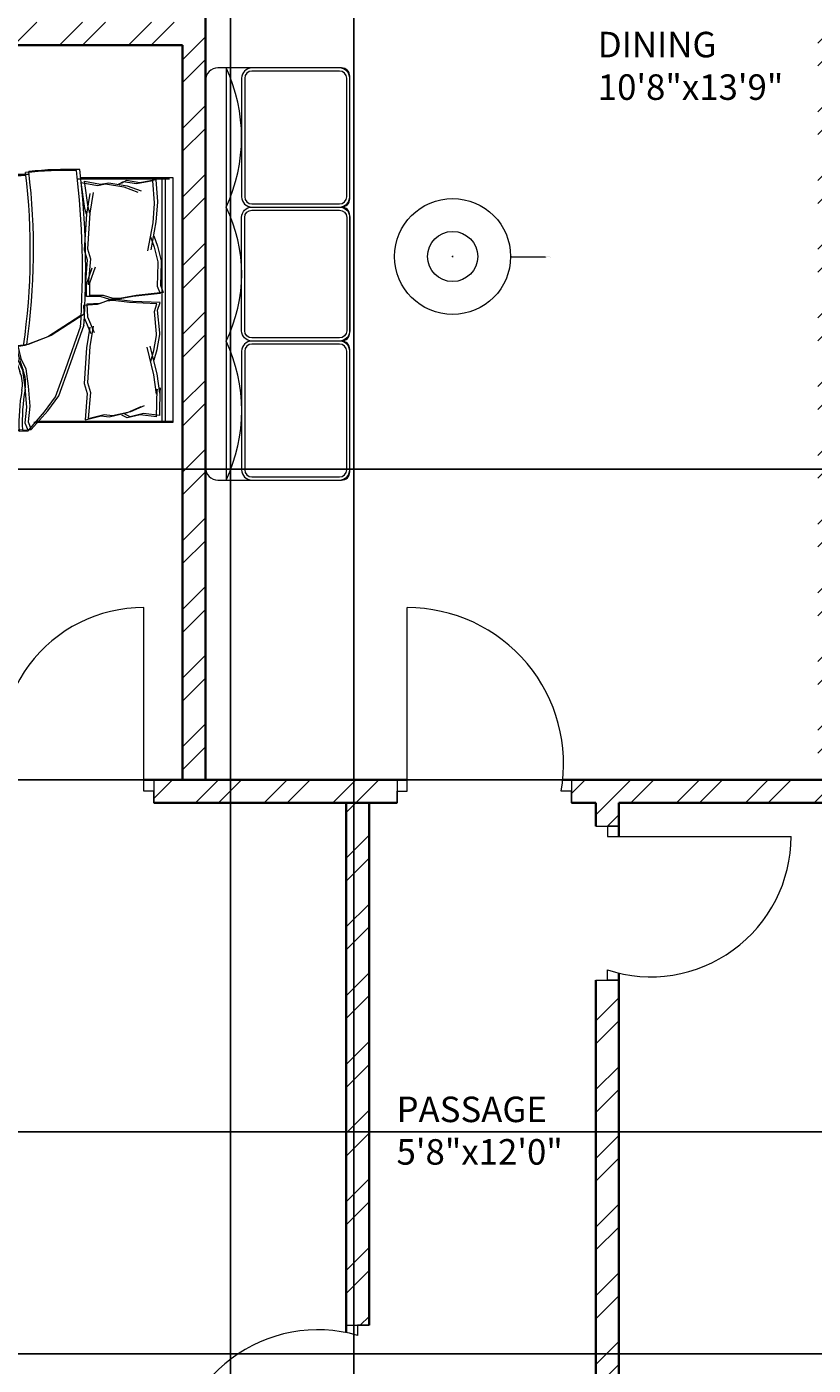
# Model space of a CAD drawing. Units: inches. Extents: x 1965 to 2673, y 1802 to 2669.
# Tile 8 of 16: x 2218 to 2372, y 2154 to 2416. Entities that reach past the tile are written whole.
import ezdxf

# ---------------------------------------------------------------- set-up
doc = ezdxf.new("R2010")
doc.units = ezdxf.units.IN
for name, color, linetype, lineweight in [('A-ANNO-DIMS', 2, 'Continuous', 18), ('A-AREA-IDEN', 7, 'Continuous', 18), ('A-DOOR', 11, 'Continuous', 18), ('A-FURN', 8, 'Continuous', 13), ('A-WALL', 7, 'Continuous', 35), ('A-WALL-PATT', 252, 'Continuous', 13)]:
    doc.layers.add(name, color=color, linetype=linetype, lineweight=lineweight)
doc.styles.get("Standard").update_dxf_attribs({"font": 'arial.ttf'})
doc.dimstyles.get("Standard").update_dxf_attribs({"dimtxt": 0.18, "dimasz": 0.18, "dimexe": 0.18, "dimexo": 0.0625, "dimgap": 0.09, "dimtad": 0, "dimtih": 1, "dimtoh": 1, "dimdec": 4, "dimzin": 0, "dimdsep": 46, "dimtxsty": 'Standard', "dimcen": 0.09, "dimadec": 0, "dimazin": 0, "dimtfac": 1, "dimtdec": 4, "dimtofl": 0, "dimtmove": 0, "dimatfit": 3, "dimfxl": 1, "dimtolj": 1, "dimtzin": 0, "dimarcsym": 0})

# ---------------------------------------------------------------- blocks, each defined once
blk = doc.blocks.new('BED-DOUBLE')
for p, q in [((3.47, 63.33), (3.47, 81.44)), ((3.47, 63.33), (3.47, 81.44)), ((3.47, 81.44), (51.49, 81.44)), ((51.26, 81.44), (51.26, 54.83)), ((51.26, 81.44), (51.26, 54.83)), ((51.49, 81.44), (51.49, 80.8)), ((3.47, 79.91), (51.26, 79.91)), ((3.47, 79.91), (51.26, 79.91)), ((3.7, 62.69), (3.7, 80.8)), ((3.7, 62.69), (3.7, 80.8)), ((3.7, 79.27), (51.49, 79.27)), ((3.7, 79.27), (51.49, 79.27)), ((16.87, 78.41), (19.76, 79.14)), ((16.87, 78.41), (19.76, 79.14)), ((19.76, 79.14), (20.09, 79.14)), ((19.76, 79.14), (20.09, 79.14)), ((20.09, 79.14), (24.53, 78.99)), ((20.09, 79.14), (24.53, 78.99)), ((24.53, 78.99), (25.98, 79.57)), ((24.53, 78.99), (25.98, 79.57)), ((24.76, 78.35), (26.21, 78.93)), ((24.76, 78.35), (26.21, 78.93)), ((25.98, 79.57), (26.56, 74.22)), ((25.98, 79.57), (26.56, 74.22)), ((26.21, 78.93), (26.78, 73.58)), ((26.21, 78.93), (26.78, 73.58)), ((27.97, 78.95), (27.73, 73.57)), ((27.97, 78.95), (27.73, 73.57)), ((29.45, 78.46), (27.97, 78.95)), ((29.45, 78.46), (27.97, 78.95)), ((33.88, 78.88), (29.45, 78.46)), ((33.88, 78.88), (29.45, 78.46)), ((34.2, 78.9), (33.88, 78.88)), ((34.2, 78.9), (33.88, 78.88)), ((37.13, 78.36), (34.2, 78.9)), ((37.13, 78.36), (34.2, 78.9)), ((45.71, 78.9), (41.91, 78.37)), ((45.71, 78.9), (41.91, 78.37)), ((50.11, 78.88), (44.7, 78.98)), ((44.7, 78.98), (45.71, 78.9)), ((50.11, 78.88), (44.7, 78.98)), ((44.7, 78.98), (45.71, 78.9)), ((50.11, 78.88), (49.73, 75.67)), ((50.11, 78.88), (49.73, 75.67)), ((51.49, 80.8), (51.49, 54.19)), ((51.49, 80.8), (51.49, 54.19)), ((3.89, 78.1), (8.17, 78.43)), ((3.89, 78.1), (8.17, 78.43)), ((3.89, 78.12), (4.47, 74.94)), ((3.89, 78.12), (4.47, 74.94)), ((4.12, 77.46), (8.4, 77.79)), ((4.12, 77.46), (8.4, 77.79)), ((4.12, 77.49), (4.7, 74.3)), ((4.12, 77.49), (4.7, 74.3)), ((8.17, 78.43), (8.28, 78.41)), ((8.17, 78.43), (8.28, 78.41)), ((8.28, 78.41), (12.1, 78.12)), ((8.28, 78.41), (12.1, 78.12)), ((8.4, 77.79), (8.51, 77.77)), ((8.4, 77.79), (8.51, 77.77)), ((8.51, 77.77), (12.33, 77.49)), ((8.51, 77.77), (12.33, 77.49)), ((12.1, 78.12), (17.6, 77.11)), ((12.1, 78.12), (17.6, 77.11)), ((12.33, 77.49), (17.82, 76.47)), ((12.33, 77.49), (17.82, 76.47)), ((14.85, 77.69), (16.87, 78.41)), ((14.85, 77.69), (16.87, 78.41)), ((15.08, 77.05), (17.1, 77.77)), ((15.08, 77.05), (17.1, 77.77)), ((17.1, 77.77), (19.99, 78.5)), ((17.1, 77.77), (19.99, 78.5)), ((19.99, 78.5), (20.31, 78.5)), ((19.99, 78.5), (20.31, 78.5)), ((20.31, 78.5), (24.76, 78.35)), ((20.31, 78.5), (24.76, 78.35)), ((28.2, 78.31), (27.96, 72.93)), ((28.2, 78.31), (27.96, 72.93)), ((29.68, 77.82), (28.2, 78.31)), ((29.68, 77.82), (28.2, 78.31)), ((34.11, 78.24), (29.68, 77.82)), ((34.11, 78.24), (29.68, 77.82)), ((34.43, 78.26), (34.11, 78.24)), ((34.43, 78.26), (34.11, 78.24)), ((37.36, 77.72), (34.43, 78.26)), ((37.36, 77.72), (34.43, 78.26)), ((41.91, 78.37), (36.49, 77.02)), ((41.91, 78.37), (36.49, 77.02)), ((42.14, 77.73), (36.72, 76.38)), ((42.14, 77.73), (36.72, 76.38)), ((39.2, 77.77), (37.13, 78.36)), ((39.19, 77.77), (37.13, 78.36)), ((39.42, 77.13), (37.36, 77.72)), ((39.42, 77.13), (37.36, 77.72)), ((45.94, 78.26), (42.14, 77.73)), ((45.94, 78.26), (42.14, 77.73)), ((50.34, 78.24), (44.93, 78.34)), ((44.93, 78.34), (45.94, 78.26)), ((50.34, 78.24), (44.93, 78.34)), ((44.93, 78.34), (45.94, 78.26)), ((50.34, 78.24), (49.96, 75.03)), ((50.34, 78.24), (49.96, 75.03)), ((4.47, 74.94), (4.03, 72.34)), ((4.47, 74.94), (4.03, 72.34)), ((4.7, 74.3), (4.26, 71.7)), ((4.7, 74.3), (4.26, 71.7)), ((5.05, 72.49), (6.06, 75.23)), ((5.05, 72.49), (6.06, 75.23)), ((5.27, 71.85), (6.29, 74.59)), ((5.27, 71.85), (6.29, 74.59)), ((26.56, 74.22), (27.13, 71.04)), ((26.56, 74.22), (27.13, 71.04)), ((26.78, 73.58), (27.36, 70.4)), ((26.78, 73.58), (27.36, 70.4)), ((27.73, 73.57), (27.35, 70.36)), ((27.73, 73.57), (27.35, 70.36)), ((49.3, 73.18), (48.12, 75.86)), ((49.3, 73.18), (48.12, 75.86)), ((49.53, 72.54), (48.35, 75.22)), ((49.53, 72.54), (48.35, 75.22)), ((49.73, 75.67), (50.32, 73.1)), ((49.73, 75.67), (50.32, 73.1)), ((49.96, 75.03), (50.55, 72.46)), ((49.96, 75.03), (50.55, 72.46)), ((4.03, 72.34), (4.61, 71.33)), ((4.03, 72.34), (4.61, 71.33)), ((4.26, 71.7), (4.84, 70.69)), ((4.26, 71.7), (4.84, 70.69)), ((4.47, 68.87), (5.05, 72.49)), ((4.47, 68.87), (5.05, 72.49)), ((4.7, 68.23), (5.27, 71.85)), ((4.7, 68.23), (5.27, 71.85)), ((27.13, 71.04), (27.13, 69.74)), ((27.13, 71.04), (27.13, 69.74)), ((27.96, 72.93), (27.58, 69.72)), ((27.96, 72.93), (27.58, 69.72)), ((50.11, 69.61), (49.3, 73.18)), ((50.11, 69.61), (49.3, 73.18)), ((50.34, 68.97), (49.53, 72.54)), ((50.34, 68.97), (49.53, 72.54)), ((50.32, 73.1), (49.81, 72.06)), ((50.32, 73.1), (49.81, 72.06)), ((50.55, 72.46), (50.04, 71.42)), ((50.55, 72.46), (50.04, 71.42)), ((4.76, 67.28), (4.47, 68.87)), ((4.76, 67.28), (4.47, 68.87)), ((4.99, 66.64), (4.7, 68.23)), ((4.99, 66.64), (4.7, 68.23)), ((27.13, 69.74), (26.56, 67.86)), ((27.13, 69.74), (26.56, 67.86)), ((27.36, 69.1), (26.78, 67.22)), ((27.36, 69.1), (26.78, 67.22)), ((27.35, 70.36), (27.43, 69.06)), ((27.35, 70.36), (27.43, 69.06)), ((27.36, 70.4), (27.36, 69.1)), ((27.36, 70.4), (27.36, 69.1)), ((27.43, 69.06), (28.13, 67.22)), ((27.43, 69.06), (28.13, 67.22)), ((27.58, 69.72), (27.66, 68.42)), ((27.58, 69.72), (27.66, 68.42)), ((27.66, 68.42), (28.35, 66.58)), ((27.66, 68.42), (28.35, 66.58)), ((49.92, 68.01), (50.11, 69.61)), ((49.92, 68.01), (50.11, 69.61)), ((50.15, 67.37), (50.34, 68.97)), ((50.15, 67.37), (50.34, 68.97)), ((4.18, 64.1), (4.76, 67.28)), ((4.18, 64.1), (4.76, 67.28)), ((4.41, 63.46), (4.99, 66.64)), ((4.41, 63.46), (4.99, 66.64)), ((6.38, 65.81), (10.41, 65.15)), ((6.38, 65.81), (10.41, 65.15)), ((24.1, 65.18), (20.95, 66.27)), ((24.1, 65.18), (20.95, 66.27)), ((24.33, 64.54), (21.18, 65.63)), ((24.33, 64.54), (21.18, 65.63)), ((26.56, 67.86), (26.56, 65.18)), ((26.56, 67.86), (26.56, 65.18)), ((26.78, 67.22), (26.78, 64.54)), ((26.78, 67.22), (26.78, 64.54)), ((28.13, 67.22), (28.29, 64.55)), ((28.13, 67.22), (28.29, 64.55)), ((28.35, 66.58), (28.52, 63.91)), ((28.35, 66.58), (28.52, 63.91)), ((30.75, 64.7), (33.82, 65.99)), ((30.75, 64.7), (33.82, 65.99)), ((32.56, 65.81), (36.59, 65.15)), ((32.56, 65.81), (36.59, 65.15)), ((50.69, 64.87), (49.92, 68.01)), ((50.69, 64.87), (49.92, 68.01)), ((50.92, 64.23), (50.15, 67.37)), ((50.92, 64.23), (50.15, 67.37)), ((9.28, 64.82), (4.18, 64.1)), ((9.28, 64.82), (4.18, 64.1)), ((9.5, 64.18), (4.41, 63.46)), ((9.5, 64.18), (4.41, 63.46)), ((6.6, 65.17), (10.64, 64.51)), ((6.61, 65.17), (10.64, 64.51)), ((10.41, 65.15), (9.28, 64.82)), ((10.41, 65.15), (9.28, 64.82)), ((10.64, 64.51), (9.5, 64.18)), ((10.64, 64.51), (9.5, 64.18)), ((10.41, 65.15), (17.42, 64.71)), ((10.41, 65.15), (17.42, 64.71)), ((10.64, 64.51), (17.65, 64.08)), ((10.64, 64.51), (17.65, 64.08)), ((17.42, 64.71), (19.38, 65.27)), ((17.42, 64.71), (19.38, 65.27)), ((17.65, 64.08), (19.61, 64.63)), ((17.65, 64.08), (19.61, 64.63)), ((19.38, 65.27), (24.51, 64.87)), ((19.38, 65.27), (24.51, 64.87)), ((19.61, 64.63), (24.74, 64.23)), ((19.61, 64.63), (24.74, 64.23)), ((26.56, 65.18), (24.1, 65.18)), ((26.56, 65.18), (24.1, 65.18)), ((26.78, 64.54), (24.33, 64.54)), ((26.78, 64.54), (24.33, 64.54)), ((28.29, 64.55), (30.75, 64.7)), ((28.29, 64.55), (30.75, 64.7)), ((28.52, 63.91), (30.97, 64.06)), ((28.52, 63.91), (30.97, 64.06)), ((30.25, 64.06), (34.44, 57.56)), ((30.25, 64.06), (34.44, 57.56)), ((30.48, 63.42), (34.67, 56.92)), ((30.48, 63.42), (34.67, 56.92)), ((30.97, 64.06), (34.04, 65.35)), ((30.97, 64.06), (34.04, 65.35)), ((40.64, 61.12), (32.3, 64.06)), ((40.64, 61.12), (32.3, 64.06)), ((40.87, 60.48), (32.53, 63.42)), ((40.87, 60.48), (32.53, 63.42)), ((32.79, 65.17), (36.82, 64.51)), ((32.79, 65.17), (36.82, 64.51)), ((36.59, 65.15), (43.6, 64.71)), ((36.59, 65.15), (43.6, 64.71)), ((36.82, 64.51), (43.83, 64.08)), ((36.82, 64.51), (43.83, 64.08)), ((43.6, 64.71), (45.56, 65.27)), ((43.6, 64.71), (45.56, 65.27)), ((43.83, 64.08), (45.79, 64.63)), ((43.83, 64.08), (45.79, 64.63)), ((45.56, 65.27), (50.69, 64.87)), ((45.56, 65.27), (50.69, 64.87)), ((45.79, 64.63), (50.92, 64.23)), ((45.79, 64.63), (50.92, 64.23)), ((46.21, 59.11), (40.64, 61.12)), ((46.21, 59.11), (40.64, 61.12)), ((46.44, 58.47), (40.87, 60.48)), ((46.44, 58.47), (40.87, 60.48)), ((49.16, 56.95), (46.21, 59.11)), ((49.16, 56.95), (46.21, 59.11)), ((49.39, 56.31), (46.44, 58.47)), ((49.39, 56.31), (46.44, 58.47)), ((34.44, 57.56), (36.15, 53.08)), ((34.44, 57.56), (36.15, 53.08)), ((34.67, 56.92), (36.38, 52.44)), ((34.67, 56.92), (36.38, 52.44)), ((52.86, 53.69), (49.16, 56.95)), ((52.86, 53.69), (49.16, 56.95)), ((53.09, 53.06), (49.39, 56.31)), ((53.09, 53.06), (49.39, 56.31)), ((36.15, 53.08), (36.46, 51.06)), ((36.15, 53.08), (36.46, 51.06)), ((38.94, 51.68), (40.95, 52.61)), ((38.94, 51.68), (40.95, 52.61)), ((40.95, 52.61), (44.36, 53.08)), ((40.95, 52.61), (44.36, 53.08)), ((44.36, 53.08), (48.23, 53.39)), ((44.36, 53.08), (48.23, 53.39)), ((44.58, 52.44), (48.46, 52.75)), ((44.58, 52.44), (48.46, 52.75)), ((48.23, 53.39), (51.33, 53.08)), ((48.23, 53.39), (51.33, 53.08)), ((48.46, 52.75), (51.55, 52.44)), ((48.46, 52.75), (51.55, 52.44)), ((51.33, 53.08), (52.86, 53.69)), ((51.33, 53.08), (52.86, 53.69)), ((51.55, 52.44), (53.09, 53.06)), ((51.55, 52.44), (53.09, 53.06)), ((52.94, 51.95), (52.86, 53.69, 3.87)), ((52.94, 51.95), (52.86, 53.69, 3.87)), ((53.17, 51.31), (53.09, 53.06, 3.87)), ((53.17, 51.31), (53.09, 53.06, 3.87)), ((36.38, 52.44), (36.69, 50.42)), ((36.38, 52.44), (36.69, 50.42)), ((36.46, 51.06), (38.94, 51.68)), ((36.46, 51.06), (38.94, 51.68)), ((36.69, 50.42), (39.16, 51.04)), ((36.69, 50.42), (39.16, 51.04)), ((39.16, 51.04), (41.18, 51.97)), ((39.16, 51.04), (41.18, 51.97)), ((41.18, 51.97), (44.58, 52.44)), ((41.18, 51.97), (44.58, 52.44)), ((15.06, 2.2), (39.67, 2.2)), ((15.06, 2.2), (39.67, 2.2)), ((15.29, 1.56), (39.9, 1.56)), ((15.29, 1.56), (39.9, 1.56))]:
    blk.add_line(p, q)
for centre, radius, start, end in [((85.16, 61.34), 83.31, 178.7218, 185.604), ((85.16, 61.34), 83.31, 178.7218, 185.604), ((21.35, -100.61), 164.97, 86.0865, 96.7821), ((21.35, -100.61), 164.97, 86.0865, 96.7821), ((21.58, -101.25), 164.97, 86.0865, 96.7821), ((21.58, -101.25), 164.97, 86.0865, 96.7821), ((85.39, 60.71), 83.31, 178.7218, 185.604), ((85.38, 60.71), 83.31, 178.7218, 185.604), ((17.75, -74.88), 129.02, 81.7845, 96.9006), ((17.75, -74.88), 129.02, 81.7845, 96.9006), ((17.98, -75.51), 129.02, 81.7845, 96.9006), ((17.98, -75.51), 129.02, 81.7845, 96.9006), ((-167.31, 50.27), 170.11, 358.4762, 1.0082), ((-167.31, 50.27), 170.11, 358.4762, 1.0082), ((-167.08, 49.63), 170.11, 358.4762, 1.0082), ((-167.08, 49.63), 170.11, 358.4762, 1.0082), ((43.74, 46.37), 6.22, 78.6608, 113.7384), ((43.74, 46.37), 6.22, 78.6608, 113.7384), ((51.32, 88.1), 36.18, 259.8763, 272.5657), ((51.32, 88.1), 36.18, 259.8763, 272.5657), ((36.63, 51), 0.185, 160.2464, 271.1377), ((36.63, 51), 0.185, 160.2464, 271.1377), ((31.15, 79.96), 29.65, 280.6617, 289.8806), ((31.15, 79.96), 29.65, 280.6617, 289.8806), ((36.86, 50.36), 0.185, 160.2464, 271.1377), ((36.86, 50.36), 0.185, 160.2464, 271.1377), ((31.38, 79.32), 29.65, 280.6617, 289.8806), ((31.38, 79.32), 29.65, 280.6617, 289.8806), ((43.97, 45.74), 6.22, 78.6608, 113.7384), ((43.97, 45.74), 6.22, 78.6608, 113.7384), ((51.55, 87.46), 36.18, 259.8763, 272.5657), ((51.55, 87.46), 36.18, 259.8763, 272.5657), ((182.26, 45.13), 129.5, 176.9791, 183.8365), ((182.26, 45.13), 129.5, 176.9791, 183.8365), ((182.49, 44.49), 129.5, 176.9791, 183.8365), ((182.49, 44.49), 129.5, 176.9791, 183.8365), ((484.82, 30.83), 482.31, 178.2277, 181.7185), ((484.82, 30.83), 482.31, 178.2277, 181.7185), ((485.05, 30.19), 482.31, 178.2277, 181.7185), ((485.05, 30.19), 482.31, 178.2277, 181.7185), ((-4508.75, 13.62), 4561.86, 0.00217, 0.28689), ((-4508.75, 13.62), 4561.86, 0.00217, 0.28689), ((-4508.52, 12.98), 4561.86, 0.00217, 0.28689), ((-4508.52, 12.98), 4561.86, 0.00217, 0.28689), ((-26.9, 16.93), 29.63, 346.0648, 358.9113), ((-26.9, 16.93), 29.63, 346.0648, 358.9113), ((-26.68, 16.29), 29.63, 346.0648, 358.9113), ((-26.68, 16.29), 29.63, 346.0648, 358.9113), ((76.15, 12.77), 23.07, 177.4714, 206.4681), ((76.15, 12.77), 23.07, 177.4714, 206.4681), ((76.38, 12.14), 23.07, 177.4714, 206.4681), ((76.38, 12.14), 23.07, 177.4714, 206.4681), ((-21.66, 11.17), 23.56, 337.9751, 356.652), ((-21.66, 11.17), 23.56, 337.9751, 356.652), ((-21.44, 10.53), 23.56, 337.9751, 356.652), ((-21.44, 10.53), 23.56, 337.9751, 356.652), ((-17.23, 105.15), 106.46, 283.3832, 287.7053), ((-17.23, 105.15), 106.46, 283.3832, 287.7053), ((-17, 104.51), 106.46, 283.3832, 287.7053), ((-17, 104.51), 106.46, 283.3832, 287.7053), ((1.08, 1.72), 1.09, 146.1736, 293.4781), ((1.08, 1.72), 1.09, 146.1736, 293.4781), ((1.31, 1.08), 1.09, 146.1736, 293.4781), ((1.31, 1.08), 1.09, 146.1736, 293.4781), ((21.42, -119.4), 121.76, 92.9958, 99.4091), ((21.42, -119.4), 121.76, 92.9958, 99.4091), ((21.65, -120.04), 121.76, 92.9958, 99.4091), ((21.65, -120.04), 121.76, 92.9958, 99.4091), ((41.15, -130.84), 133.04, 84.4998, 90.6351), ((41.15, -130.84), 133.04, 84.4998, 90.6351), ((41.38, -131.48), 133.04, 84.4998, 90.6351), ((41.37, -131.48), 133.04, 84.4998, 90.6351), ((54.4, 2.57), 1.1, 242.6588, 356.02), ((54.4, 2.57), 1.1, 242.6588, 356.02), ((54.63, 1.93), 1.1, 242.6588, 356.02), ((54.63, 1.93), 1.1, 242.6588, 356.02)]:
    blk.add_arc(centre, radius, start, end)
blk = doc.blocks.new('*D47')
at = {"layer": 'A-ANNO-DIMS', "color": 0, "lineweight": -2, "transparency": 16777216}
for p, q in [((2573.53, 2199.58), (2012.19, 2199.58)), ((2012.37, 2199.4), (2012.37, 2178.02)), ((2012.37, 2156.27), (2012.37, 2177.65)), ((2573.53, 2156.09), (2012.19, 2156.09))]:
    blk.add_line(p, q, dxfattribs=at)
at = {"layer": 'A-ANNO-DIMS', "color": 0, "transparency": 16777216}
for points in [[(2012.34, 2199.4), (2012.4, 2199.4), (2012.37, 2199.58)], [(2012.34, 2156.27), (2012.4, 2156.27), (2012.37, 2156.09)]]:
    blk.add_solid(points, dxfattribs=at)
at = {"layer": 'Defpoints', "color": 0, "transparency": 16777216}
for p in [(2012.37, 2199.58), (2573.59, 2199.58), (2573.59, 2156.09)]:
    blk.add_point(p, dxfattribs=at)
at = {"layer": 'A-ANNO-DIMS', "color": 0, "transparency": 16777216, "insert": (2012.37, 2177.83), "char_height": 0.18, "attachment_point": 5}
blk.add_mtext('\\A1;43.48', dxfattribs=at)
blk = doc.blocks.new('*D48')
at = {"layer": 'A-ANNO-DIMS', "color": 0, "lineweight": -2, "transparency": 16777216}
for p, q in [((2573.53, 2329.47), (2012.19, 2329.47)), ((2012.37, 2329.29), (2012.37, 2299.21)), ((2012.37, 2268.77), (2012.37, 2298.85)), ((2573.53, 2268.59), (2012.19, 2268.59))]:
    blk.add_line(p, q, dxfattribs=at)
at = {"layer": 'A-ANNO-DIMS', "color": 0, "transparency": 16777216}
for points in [[(2012.34, 2329.29), (2012.4, 2329.29), (2012.37, 2329.47)], [(2012.34, 2268.77), (2012.4, 2268.77), (2012.37, 2268.59)]]:
    blk.add_solid(points, dxfattribs=at)
at = {"layer": 'Defpoints', "color": 0, "transparency": 16777216}
for p in [(2012.37, 2329.47), (2573.59, 2329.47), (2573.59, 2268.59)]:
    blk.add_point(p, dxfattribs=at)
at = {"layer": 'A-ANNO-DIMS', "color": 0, "transparency": 16777216, "insert": (2012.37, 2299.03), "char_height": 0.18, "attachment_point": 5}
blk.add_mtext('\\A1;60.87', dxfattribs=at)
blk = doc.blocks.new('*D53')
at = {"layer": 'A-ANNO-DIMS', "color": 0, "lineweight": -2, "transparency": 16777216}
for p, q in [((2257.52, 2457.53), (2257.52, 1838.49)), ((2281.66, 2457.53), (2281.66, 1838.49)), ((2257.7, 1838.67), (2269.12, 1838.67)), ((2281.48, 1838.67), (2270.05, 1838.67))]:
    blk.add_line(p, q, dxfattribs=at)
at = {"layer": 'A-ANNO-DIMS', "color": 0, "transparency": 16777216}
for points in [[(2257.7, 1838.7), (2257.7, 1838.64), (2257.52, 1838.67)], [(2281.48, 1838.7), (2281.48, 1838.64), (2281.66, 1838.67)]]:
    blk.add_solid(points, dxfattribs=at)
at = {"layer": 'Defpoints', "color": 0, "transparency": 16777216}
for p in [(2257.52, 2457.59), (2281.66, 2457.59), (2281.66, 1838.67)]:
    blk.add_point(p, dxfattribs=at)
at = {"layer": 'A-ANNO-DIMS', "color": 0, "transparency": 16777216, "insert": (2269.59, 1838.67), "char_height": 0.18, "attachment_point": 5}
blk.add_mtext('\\A1;24.145', dxfattribs=at)
blk = doc.blocks.new('*D55')
at = {"layer": 'A-ANNO-DIMS', "color": 0, "lineweight": -2, "transparency": 16777216}
for p, q in [((2300.93, 2371.16), (2301.11, 2371.16)), ((2301.02, 2371.07), (2301.02, 2371.25)), ((2319.19, 2371.06), (2312.55, 2371.1))]:
    blk.add_line(p, q, dxfattribs=at)
at = {"layer": 'A-ANNO-DIMS', "color": 0, "transparency": 16777216}
blk.add_solid([(2312.56, 2371.13), (2312.55, 2371.07), (2312.37, 2371.1)], dxfattribs=at)
at = {"layer": 'Defpoints', "color": 0, "transparency": 16777216}
for p in [(2289.66, 2371.22), (2312.37, 2371.1)]:
    blk.add_point(p, dxfattribs=at)
at = {"layer": 'A-ANNO-DIMS', "color": 0, "transparency": 16777216, "insert": (2319.75, 2371.06), "char_height": 0.18, "attachment_point": 5}
blk.add_mtext('\\A1;∅22.716', dxfattribs=at)

msp = doc.modelspace()

# ---------------------------------------------------------------- hatches: boundary and pattern name
at = {"layer": 'A-WALL-PATT'}
h = msp.add_hatch(dxfattribs=at)
h.set_pattern_fill('ANSI32', color=256)
h.paths.add_polyline_path([(2051.5927, 2561.0914), (2076.7559, 2561.0914), (2076.7559, 2563.3414), (2076.7559, 2565.5914), (2047.0927, 2565.5914), (2047.0927, 2518.3824), (2051.5927, 2518.3824)])
h.paths.add_polyline_path([(2051.5927, 2458.3824), (2049.3427, 2458.3824), (2047.0927, 2458.3824), (2047.0927, 2412.5914), (2248.0927, 2412.5914), (2248.0927, 2268.5914), (2252.5927, 2268.5914), (2252.5927, 2412.5914), (2252.5927, 2421.0404), (2250.3427, 2421.0404), (2248.0927, 2421.0404), (2248.0927, 2417.0914), (2051.5927, 2417.0914)])
h.paths.add_polyline_path([(2211.4933, 2268.5914), (2104.0927, 2268.5914), (2104.0927, 2272.4654), (2101.8427, 2272.4654), (2099.5927, 2272.4654), (2099.5927, 2268.5914), (2051.5927, 2268.5914), (2051.5927, 2264.0914), (2147.5927, 2264.0914), (2147.5927, 2259.8893), (2152.0927, 2259.8893), (2152.0927, 2264.0914), (2211.4933, 2264.0914), (2211.4933, 2266.3414)])
h.paths.add_polyline_path([(2104.0927, 2376.0914), (2099.5927, 2376.0914), (2047.0927, 2376.0914), (2047.0927, 2333.0682), (2051.5927, 2333.0682), (2051.5927, 2371.5914), (2099.5927, 2371.5914), (2099.5927, 2293.6123), (2104.0927, 2293.6123)], flags=17)
h.paths.add_polyline_path([(2051.5927, 2309.0682), (2047.0927, 2309.0682), (2047.0927, 2233.5821), (2051.5927, 2233.5821)])
h.paths.add_polyline_path([(2104.0927, 2412.5914), (2099.5927, 2412.5914), (2099.5927, 2376.0914), (2104.0927, 2376.0914)], flags=17)
h.paths.add_polyline_path([(2290.1254, 2268.5914), (2242.4924, 2268.5914), (2242.4924, 2264.0914), (2290.1254, 2264.0914), (2290.1254, 2266.3414)])
h.paths.add_polyline_path([(2284.653, 2264.0914), (2280.153, 2264.0914), (2280.153, 2161.6826), (2284.653, 2161.6826)])
h.paths.add_polyline_path([(2578.0927, 2329.4656), (2573.5927, 2329.4656), (2573.5927, 2268.5914), (2525.5927, 2268.5914), (2525.5927, 2271.9222), (2523.3427, 2271.9222), (2521.0927, 2271.9222), (2521.0927, 2268.5914), (2324.2835, 2268.5914), (2324.2835, 2264.0914), (2329.0927, 2264.0914), (2329.0927, 2259.4977), (2333.5927, 2259.4977), (2333.5927, 2264.0914), (2473.0927, 2264.0914), (2473.0927, 2259.9371), (2477.5927, 2259.9371), (2477.5927, 2264.0914), (2573.5927, 2264.0914), (2573.5927, 2235.5751), (2578.0927, 2235.5751)])
h.paths.add_polyline_path([(2377.0927, 2412.5914), (2578.0927, 2412.5914), (2578.0927, 2444.2286), (2575.8427, 2444.2286), (2573.5927, 2444.2286), (2573.5927, 2417.0914), (2429.5927, 2417.0914), (2377.0927, 2417.0914), (2377.0927, 2421.7443), (2372.5927, 2421.7443), (2372.5927, 2268.5914), (2377.0927, 2268.5914)])
h.paths.add_polyline_path([(2525.5927, 2371.5914), (2573.5927, 2371.5914), (2573.5927, 2353.4656), (2578.0927, 2353.4656), (2578.0927, 2376.0914), (2525.5927, 2376.0914), (2521.0927, 2376.0914), (2521.0927, 2290.6472), (2525.5927, 2290.6472)], flags=17)
h.paths.add_polyline_path([(2477.5927, 2236.4106), (2475.3427, 2236.4106), (2473.0927, 2236.4106), (2473.0927, 2084.5914), (2465.3309, 2084.5914), (2465.3309, 2080.0914), (2481.6764, 2080.0914), (2481.6764, 2082.3414), (2481.6764, 2084.5914), (2477.5927, 2084.5914), (2477.5927, 2151.5914), (2573.5927, 2151.5914), (2573.5927, 2130.2907), (2578.0927, 2130.2907), (2578.0927, 2199.5751), (2575.8427, 2199.5751), (2573.5927, 2199.5751), (2573.5927, 2156.0914), (2477.5927, 2156.0914)])
h.paths.add_polyline_path([(2573.5927, 2084.5914), (2505.5513, 2084.5914), (2505.5513, 2080.0914), (2573.5927, 2080.0914)], flags=17)
h.paths.add_polyline_path([(2578.0927, 2106.2907), (2575.8427, 2106.2907), (2573.5927, 2106.2907), (2573.5927, 2050.8986), (2578.0927, 2050.8986)])
h.paths.add_polyline_path([(2578.0927, 1990.8986), (2575.8427, 1990.8986), (2573.5927, 1990.8986), (2573.5927, 1936.0914), (2522.132, 1936.0914), (2522.132, 1931.5914), (2578.0927, 1931.5914)])
h.paths.add_polyline_path([(2462.132, 1936.0914), (2429.5927, 1936.0914), (2429.5927, 2080.0914), (2432.623, 2080.0914), (2432.623, 2082.3414), (2432.623, 2084.5914), (2429.5927, 2084.5914), (2429.5927, 2120.5914), (2333.5927, 2120.5914), (2333.5927, 2229.3125), (2331.3427, 2229.3125), (2329.0927, 2229.3125), (2329.0927, 2116.0914), (2425.0927, 2116.0914), (2425.0927, 1936.0914), (2346.4058, 1936.0914), (2346.4058, 1931.5914), (2462.132, 1931.5914), (2462.132, 1933.8414)])
h.paths.add_polyline_path([(2211.767, 1933.8414), (2211.767, 1936.0914), (2200.0927, 1936.0914), (2200.0927, 2080.0914), (2200.0927, 2116.0914), (2284.653, 2116.0914), (2284.653, 2130.591), (2282.403, 2130.591), (2280.153, 2130.591), (2280.153, 2120.5914), (2200.0927, 2120.5914), (2195.5927, 2120.5914), (2195.5927, 2080.0914), (2195.5927, 1936.0914), (2139.0533, 1936.0914), (2139.0533, 1931.5914), (2211.767, 1931.5914)])
h.paths.add_polyline_path([(2282.2502, 1933.8414), (2282.2502, 1936.0914), (2259.767, 1936.0914), (2259.767, 1931.5914), (2282.2502, 1931.5914)], flags=17)
h.paths.add_polyline_path([(2051.5927, 1987.096), (2049.3427, 1987.096), (2047.0927, 1987.096), (2047.0927, 1931.5914), (2079.0533, 1931.5914), (2079.0533, 1933.8414), (2079.0533, 1936.0914), (2051.5927, 1936.0914)])
h.paths.add_polyline_path([(2051.5927, 2197.5821), (2049.3427, 2197.5821), (2047.0927, 2197.5821), (2047.0927, 2141.952), (2051.5927, 2141.952), (2051.5927, 2151.5914), (2147.5927, 2151.5914), (2147.5927, 2084.5914), (2144.3652, 2084.5914), (2144.3652, 2080.0914), (2155.9662, 2080.0914), (2155.9662, 2082.3414), (2155.9662, 2084.5914), (2152.0927, 2084.5914), (2152.0927, 2239.4921), (2149.8427, 2239.4921), (2147.5927, 2239.4921), (2147.5927, 2156.0914), (2051.5927, 2156.0914)])
h.paths.add_polyline_path([(2051.5927, 2080.0914), (2123.8575, 2080.0914), (2123.8575, 2082.3414), (2123.8575, 2084.5914), (2051.5927, 2084.5914), (2051.5927, 2117.952), (2047.0927, 2117.952), (2047.0927, 2047.096), (2051.5927, 2047.096)])
h = msp.add_hatch(dxfattribs=at)
h.set_pattern_fill('ANSI32', color=256)
h.paths.add_polyline_path([(2210.2316, 2563.3414), (2210.2316, 2565.5914), (2136.7559, 2565.5914), (2136.7559, 2561.0914), (2195.5927, 2561.0914), (2195.5927, 2485.8604), (2200.0927, 2485.8604), (2200.0927, 2561.0914), (2210.2316, 2561.0914)])
h.paths.add_polyline_path([(2285.9734, 2565.5914), (2234.2316, 2565.5914), (2234.2316, 2561.0914), (2248.0927, 2561.0914), (2248.0927, 2462.0914), (2200.0927, 2462.0914), (2200.0927, 2465.2357), (2197.8427, 2465.2357), (2195.5927, 2465.2357), (2195.5927, 2457.5914), (2248.0927, 2457.5914), (2248.0927, 2452.628), (2252.5927, 2452.628), (2252.5927, 2457.5914), (2257.5156, 2457.5914), (2257.5156, 2459.8414), (2257.5156, 2462.0914), (2252.5927, 2462.0914), (2252.5927, 2561.0914), (2285.9734, 2561.0914)])
h.paths.add_polyline_path([(2213.1374, 1872.8885), (2461.061, 1872.8885), (2461.061, 1909.9813), (2213.1374, 1909.9813)], flags=9)
h.paths.add_polyline_path([(2328.4056, 1942.3944), (2340.6089, 1942.3944), (2340.6089, 1952.6979), (2328.4056, 1952.6979)], flags=9)
h.paths.add_polyline_path([(2353.5759, 2030.9808), (2376.6455, 2030.9808), (2376.6455, 2041.2844), (2353.5759, 2041.2844)], flags=9)
h.paths.add_polyline_path([(2289.989, 2074.1041), (2326.916, 2074.1041), (2326.916, 2092.7615), (2289.989, 2092.7615)], flags=9)
h.paths.add_polyline_path([(2497.9, 2052.8638), (2548.3741, 2052.8638), (2548.3741, 2071.5212), (2497.9, 2071.5212)], flags=9)
h.paths.add_polyline_path([(2486.59, 2116.4883), (2515.7475, 2116.4883), (2515.7475, 2135.1456), (2486.59, 2135.1456)], flags=9)
h.paths.add_polyline_path([(2497.3007, 2181.2877), (2530.459, 2181.2877), (2530.459, 2199.945), (2497.3007, 2199.945)], flags=9)
h.paths.add_polyline_path([(2288.237, 2190.3228), (2324.1238, 2190.3228), (2324.1238, 2208.9802), (2288.237, 2208.9802)], flags=9)
h.paths.add_polyline_path([(2350.806, 2127.8307), (2387.733, 2127.8307), (2387.733, 2146.488), (2350.806, 2146.488)], flags=9)
h.paths.add_polyline_path([(2530.3237, 2315.2679), (2559.5563, 2315.2679), (2559.5563, 2333.9252), (2530.3237, 2333.9252)], flags=9)
h.paths.add_polyline_path([(2418.419, 2383.4707), (2468.2894, 2383.4707), (2468.2894, 2402.1281), (2418.419, 2402.1281)], flags=9)
h.paths.add_polyline_path([(2327.4503, 2399.0281), (2364.3773, 2399.0281), (2364.3773, 2417.6854), (2327.4503, 2417.6854)], flags=9)
h.paths.add_polyline_path([(2147.9722, 2271.4601), (2197.8426, 2271.4601), (2197.8426, 2290.1174), (2147.9722, 2290.1174)], flags=9)
h.paths.add_polyline_path([(2474.3875, 2421.594), (2524.8616, 2421.594), (2524.8616, 2440.2514), (2474.3875, 2440.2514)], flags=9)
h.paths.add_polyline_path([(2063.9863, 2052.9059), (2114.4604, 2052.9059), (2114.4604, 2071.5632), (2063.9863, 2071.5632)], flags=9)
h.paths.add_polyline_path([(2200.3335, 2133.7067), (2237.2605, 2133.7067), (2237.2605, 2152.364), (2200.3335, 2152.364)], flags=9)
h.paths.add_polyline_path([(2080.5973, 2184.636), (2113.8681, 2184.636), (2113.8681, 2203.2933), (2080.5973, 2203.2933)], flags=9)
h.paths.add_polyline_path([(2102.4918, 2116.4497), (2131.6494, 2116.4497), (2131.6494, 2135.107), (2102.4918, 2135.107)], flags=9)
h.paths.add_polyline_path([(2056.2753, 2308.5576), (2085.5079, 2308.5576), (2085.5079, 2327.2149), (2056.2753, 2327.2149)], flags=9)
h.paths.add_polyline_path([(2385.619, 2500.9729), (2414.8516, 2500.9729), (2414.8516, 2519.6303), (2385.619, 2519.6303)], flags=9)
h.paths.add_polyline_path([(2286.6643, 2508.6826), (2320.0715, 2508.6826), (2320.0715, 2527.34), (2286.6643, 2527.34)], flags=9)
h.paths.add_polyline_path([(2206.5604, 2500.7243), (2235.793, 2500.7243), (2235.793, 2519.3817), (2206.5604, 2519.3817)], flags=25)
h.paths.add_polyline_path([(2062.6644, 2424.4027), (2112.5348, 2424.4027), (2112.5348, 2443.0601), (2062.6644, 2443.0601)], flags=9)
h = msp.add_hatch(dxfattribs=at)
h.set_pattern_fill('ANSI32', color=256)
h.paths.add_polyline_path([(2429.5927, 2468.6101), (2427.3427, 2468.6101), (2425.0927, 2468.6101), (2425.0927, 2462.0914), (2377.0927, 2462.0914), (2377.0927, 2561.0914), (2390.4173, 2561.0914), (2390.4173, 2565.5914), (2321.9734, 2565.5914), (2321.9734, 2561.0914), (2372.5927, 2561.0914), (2372.5927, 2462.0914), (2281.6605, 2462.0914), (2281.6605, 2457.5914), (2372.5927, 2457.5914), (2372.5927, 2451.3316), (2377.0927, 2451.3316), (2377.0927, 2457.5914), (2429.5927, 2457.5914)])
h.paths.add_polyline_path([(2480.8929, 2565.5914), (2414.4173, 2565.5914), (2414.4173, 2561.0914), (2425.0927, 2561.0914), (2425.0927, 2489.9153), (2429.5927, 2489.9153), (2429.5927, 2561.0914), (2480.8929, 2561.0914), (2480.8929, 2563.3414)])
h.paths.add_polyline_path([(2213.1374, 1872.8885), (2461.061, 1872.8885), (2461.061, 1909.9813), (2213.1374, 1909.9813)], flags=9)
h.paths.add_polyline_path([(2328.4056, 1942.3944), (2340.6089, 1942.3944), (2340.6089, 1952.6979), (2328.4056, 1952.6979)], flags=9)
h.paths.add_polyline_path([(2353.5759, 2030.9808), (2376.6455, 2030.9808), (2376.6455, 2041.2844), (2353.5759, 2041.2844)], flags=9)
h.paths.add_polyline_path([(2289.989, 2074.1041), (2326.916, 2074.1041), (2326.916, 2092.7615), (2289.989, 2092.7615)], flags=9)
h.paths.add_polyline_path([(2497.9, 2052.8638), (2548.3741, 2052.8638), (2548.3741, 2071.5212), (2497.9, 2071.5212)], flags=9)
h.paths.add_polyline_path([(2486.59, 2116.4883), (2515.7475, 2116.4883), (2515.7475, 2135.1456), (2486.59, 2135.1456)], flags=9)
h.paths.add_polyline_path([(2497.3007, 2181.2877), (2530.459, 2181.2877), (2530.459, 2199.945), (2497.3007, 2199.945)], flags=9)
h.paths.add_polyline_path([(2288.237, 2190.3228), (2324.1238, 2190.3228), (2324.1238, 2208.9802), (2288.237, 2208.9802)], flags=9)
h.paths.add_polyline_path([(2350.806, 2127.8307), (2387.733, 2127.8307), (2387.733, 2146.488), (2350.806, 2146.488)], flags=9)
h.paths.add_polyline_path([(2530.3237, 2315.2679), (2559.5563, 2315.2679), (2559.5563, 2333.9252), (2530.3237, 2333.9252)], flags=9)
h.paths.add_polyline_path([(2418.419, 2383.4707), (2468.2894, 2383.4707), (2468.2894, 2402.1281), (2418.419, 2402.1281)], flags=9)
h.paths.add_polyline_path([(2327.4503, 2399.0281), (2364.3773, 2399.0281), (2364.3773, 2417.6854), (2327.4503, 2417.6854)], flags=9)
h.paths.add_polyline_path([(2147.9722, 2271.4601), (2197.8426, 2271.4601), (2197.8426, 2290.1174), (2147.9722, 2290.1174)], flags=9)
h.paths.add_polyline_path([(2474.3875, 2421.594), (2524.8616, 2421.594), (2524.8616, 2440.2514), (2474.3875, 2440.2514)], flags=9)
h.paths.add_polyline_path([(2063.9863, 2052.9059), (2114.4604, 2052.9059), (2114.4604, 2071.5632), (2063.9863, 2071.5632)], flags=9)
h.paths.add_polyline_path([(2200.3335, 2133.7067), (2237.2605, 2133.7067), (2237.2605, 2152.364), (2200.3335, 2152.364)], flags=9)
h.paths.add_polyline_path([(2080.5973, 2184.636), (2113.8681, 2184.636), (2113.8681, 2203.2933), (2080.5973, 2203.2933)], flags=9)
h.paths.add_polyline_path([(2102.4918, 2116.4497), (2131.6494, 2116.4497), (2131.6494, 2135.107), (2102.4918, 2135.107)], flags=9)
h.paths.add_polyline_path([(2056.2753, 2308.5576), (2085.5079, 2308.5576), (2085.5079, 2327.2149), (2056.2753, 2327.2149)], flags=9)
h.paths.add_polyline_path([(2385.619, 2500.9729), (2414.8516, 2500.9729), (2414.8516, 2519.6303), (2385.619, 2519.6303)], flags=25)
h.paths.add_polyline_path([(2286.6643, 2508.6826), (2320.0715, 2508.6826), (2320.0715, 2527.34), (2286.6643, 2527.34)], flags=25)
h.paths.add_polyline_path([(2206.5604, 2500.7243), (2235.793, 2500.7243), (2235.793, 2519.3817), (2206.5604, 2519.3817)], flags=9)
h.paths.add_polyline_path([(2062.6644, 2424.4027), (2112.5348, 2424.4027), (2112.5348, 2443.0601), (2062.6644, 2443.0601)], flags=9)

# ---------------------------------------------------------------- linework, layer by layer
at = {"layer": 'A-DOOR'}
for p, q in [((2240.4924, 2266.3414), (2240.4924, 2302.3414)), ((2292.1254, 2266.3414), (2292.1254, 2302.3414)), ((2242.4924, 2268.5914), (2242.4924, 2264.0914)), ((2290.1254, 2268.5914), (2290.1254, 2264.0914)), ((2324.2835, 2268.5914), (2324.2835, 2264.0914)), ((2242.4924, 2266.3414), (2240.4924, 2266.3414)), ((2242.4924, 2264.0914), (2242.4924, 2266.3414)), ((2290.1254, 2264.0914), (2290.1254, 2266.3414)), ((2290.1254, 2266.3414), (2292.1254, 2266.3414)), ((2324.2835, 2266.3414), (2322.2835, 2266.3414)), ((2324.2835, 2264.0914), (2324.2835, 2266.3414)), ((2329.0927, 2259.4977), (2333.5927, 2259.4977)), ((2333.5927, 2259.4977), (2331.3427, 2259.4977)), ((2331.3427, 2259.4977), (2331.3427, 2257.4977)), ((2331.3427, 2257.4977), (2367.3427, 2257.4977)), ((2331.3427, 2229.3125), (2331.3427, 2231.3125)), ((2329.0927, 2229.3125), (2333.5927, 2229.3125)), ((2333.5927, 2229.3125), (2331.3427, 2229.3125)), ((2280.153, 2161.6826), (2284.653, 2161.6826)), ((2284.653, 2161.6826), (2282.403, 2161.6826)), ((2282.403, 2161.6826), (2282.403, 2159.6826)), ((2284.653, 2161.6826), (2284.653, 2161.6826))]:
    msp.add_line(p, q, dxfattribs=at)
for centre, radius, start, end in [((2240.4924, 2274.217), 28.1243, 90, 196.261997), ((2292.1254, 2271.7093), 30.6321, 349.907493, 90), ((2339.8196, 2257.4977), 27.5231, 252.0617, 0), ((2274.5969, 2132.591), 28.1938, 73.926247, 180)]:
    msp.add_arc(centre, radius, start, end, dxfattribs=at)
at = {"layer": 'A-FURN', "ltscale": 0.03}
msp.add_lwpolyline([(2280.8636, 2382.4838), (2280.8636, 2406.4942, 0.41421356), (2279.2482, 2408.1097), (2255.0159, 2408.1097, 0.41421356), (2252.5927, 2405.6865), (2252.5927, 2329.7588, 0.41421356), (2255.0159, 2327.3356), (2279.2482, 2327.3356, 0.41421356), (2280.8636, 2328.9511), (2280.8636, 2352.9615, 0.41421356), (2279.2482, 2354.577, -1), (2279.2482, 2354.6167, 0.41421356), (2280.8636, 2356.2322), (2280.8636, 2379.2131, 0.41421356), (2279.2482, 2380.8286, -1), (2279.2482, 2380.8683, 0.41421356)], format="xyb", close=True, dxfattribs=at)
at = {"layer": 'A-FURN'}
msp.add_lwpolyline([(2256.6314, 2408.1097), (2256.6314, 2327.3356)], dxfattribs=at)
for points in [[(2278.8443, 2408.1097), (2261.6798, 2408.1097, 0.41421356), (2259.6604, 2406.0904), (2259.6604, 2382.8678, 0.41421356), (2261.6798, 2380.8485), (2278.8443, 2380.8485, 0.41421356), (2280.8636, 2382.8678), (2280.8636, 2406.0904, 0.41421356)], [(2278.8443, 2407.5039), (2261.6798, 2407.5039, 0.41421356), (2260.2662, 2406.0904), (2260.2662, 2382.8678, 0.41421356), (2261.6798, 2381.4543), (2278.8443, 2381.4543, 0.41421356), (2280.2578, 2382.8678), (2280.2578, 2406.0904, 0.41421356)], [(2278.8443, 2354.5969), (2261.6798, 2354.5969, -0.41421356), (2259.6604, 2356.6162), (2259.6604, 2378.8291, -0.41421356), (2261.6798, 2380.8485), (2278.8443, 2380.8485, -0.41421356), (2280.8636, 2378.8291), (2280.8636, 2356.6162, -0.41421356)], [(2278.8443, 2355.2027), (2261.6798, 2355.2027, -0.41421356), (2260.2662, 2356.6162), (2260.2662, 2378.8291, -0.41421356), (2261.6798, 2380.2427), (2278.8443, 2380.2427, -0.41421356), (2280.2578, 2378.8291), (2280.2578, 2356.6162, -0.41421356)], [(2278.8443, 2354.5969), (2261.6798, 2354.5969, 0.41421356), (2259.6604, 2352.5775), (2259.6604, 2329.355, 0.41421356), (2261.6798, 2327.3356), (2278.8443, 2327.3356, 0.41421356), (2280.8636, 2329.355), (2280.8636, 2352.5775, 0.41421356)], [(2278.8443, 2353.9911), (2261.6798, 2353.9911, 0.41421356), (2260.2662, 2352.5775), (2260.2662, 2329.355, 0.41421356), (2261.6798, 2327.9414), (2278.8443, 2327.9414, 0.41421356), (2280.2578, 2329.355), (2280.2578, 2352.5775, 0.41421356)]]:
    msp.add_lwpolyline(points, format="xyb", close=True, dxfattribs=at)
for radius in [11.3581, 4.9166]:
    msp.add_circle((2301.0171, 2371.1611), radius, dxfattribs=at)
for centre, radius, start, end in [((2227.5191, 2394.4791), 32.1453, 334.910626, 25.089374), ((2229.875, 2367.7227), 29.8026, 333.868999, 26.131001), ((2227.8556, 2340.9662), 31.8408, 334.653824, 25.346176)]:
    msp.add_arc(centre, radius, start, end, dxfattribs=at)
at = {"layer": 'A-WALL'}
for p, q in [((2252.5927, 2421.0404), (2252.5927, 2268.5914)), ((2047.0927, 2412.5914), (2248.0927, 2412.5914)), ((2248.0927, 2412.5914), (2248.0927, 2268.5914)), ((2252.5927, 2412.5914), (2252.5927, 2268.5914)), ((2240.4924, 2268.5914), (2292.1254, 2268.5914)), ((2322.5984, 2268.5914), (2521.0927, 2268.5914)), ((2242.4924, 2264.0914), (2290.1254, 2264.0914)), ((2280.153, 2264.0914), (2280.153, 2160.2319)), ((2284.653, 2264.0914), (2284.653, 2161.6826)), ((2324.2835, 2264.0914), (2329.0927, 2264.0914)), ((2329.0927, 2264.0914), (2329.0927, 2259.4977)), ((2333.5927, 2264.0914), (2333.5927, 2257.4977)), ((2333.5927, 2264.0914), (2473.0927, 2264.0914)), ((2333.5927, 2230.6883), (2333.5927, 2120.5914)), ((2329.0927, 2229.3125), (2329.0927, 2116.0914))]:
    msp.add_line(p, q, dxfattribs=at)

# ---------------------------------------------------------------- block references
at = {"layer": 'A-FURN', "rotation": 269.9999998331858}
msp.add_blockref('BED-DOUBLE', (2164.7524, 2390.0859), dxfattribs=at)

# ---------------------------------------------------------------- texts
at = {"layer": 'A-AREA-IDEN', "char_height": 5, "attachment_point": 1}
for s, width, insert in [('DINING\\P10\'8"x13\'9"', 331.64776, (2329.4609, 2415.1974)), ('PASSAGE\\P5\'8"x12\'0"', 214.822327, (2290.0259, 2206.4921))]:
    msp.add_mtext_dynamic_manual_height_columns(s, width=width, gutter_width=12.5, heights=[0], dxfattribs=dict(at, insert=insert))

# ---------------------------------------------------------------- dimensions: what is measured, and where the dimension line sits
at = {"layer": 'A-ANNO-DIMS'}
dim = msp.add_linear_dim(base=(2281.6605, 1838.6715), p1=(2257.5156, 2457.5914), p2=(2281.6605, 2457.5914), dimstyle='Standard', override={"dimdec": 3, "dimlfac": 1, "dimrnd": 0, "dimzin": 0, "dimdsep": 46, "dimlunit": 2}, dxfattribs=at)
dim.commit()
dim.dimension.update_dxf_attribs({"geometry": '*D53', "text_midpoint": (2269.588, 1838.6715)})
dim = msp.add_diameter_dim_2p(p1=(2289.6591, 2371.2225), p2=(2312.375, 2371.0996), dimstyle='Standard', override={"dimdec": 3, "dimlfac": 1, "dimrnd": 0, "dimzin": 0, "dimdsep": 46, "dimlunit": 2}, dxfattribs=at)
dim.commit()
dim.dimension.update_dxf_attribs({"geometry": '*D55', "text_midpoint": (2319.1898, 2371.0627), "dimtype": 163})
for base, p1, p2, picture, middle in [((2012.3677, 2329.4656), (2573.5927, 2268.5914), (2573.5927, 2329.4656), '*D48', (2012.3677, 2299.0285)), ((2012.3677, 2199.5751), (2573.5927, 2156.0914), (2573.5927, 2199.5751), '*D47', (2012.3677, 2177.8332))]:
    dim = msp.add_linear_dim(base=base, p1=p1, p2=p2, angle=90, dimstyle='Standard', override={"dimdec": 2, "dimlfac": 1, "dimrnd": 0, "dimzin": 0, "dimdsep": 46, "dimlunit": 2}, dxfattribs=at)
    dim.commit()
    dim.dimension.update_dxf_attribs({"geometry": picture, "text_midpoint": middle})

doc.saveas('drawing.dxf')
